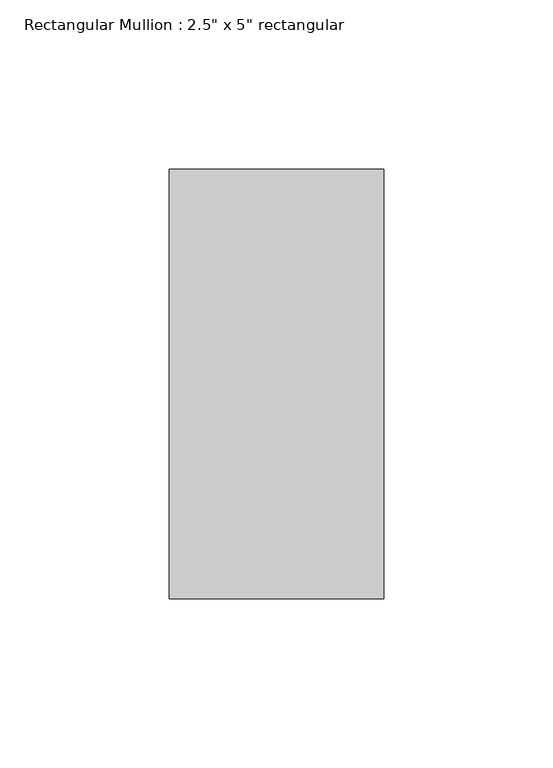
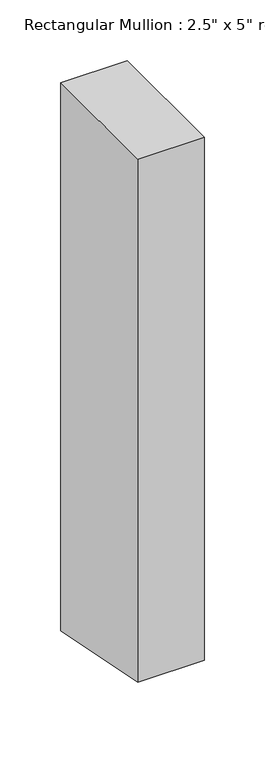
"""IFC4 building model written with IfcOpenShell, lengths in millimetres: member geometry."""

from ifc_helpers import new_model, si_unit, frame, origin, place, context, project, spatial, polyline, outline, extrude, source, transform, mapped, element, save


def member_efc2c738(model_context):
    return source(origin(), model_context, "Body", "SweptSolid", [
        extrude(outline(polyline([(-63.5, 0.0), (63.5, 0.0), (63.5, -552.0583104), (-63.5, -526.7964398), (-63.5, 0.0)])), frame((-63.5, 0.0, 0.0), z_axis=(1.0, 0.0, 0.0), x_axis=(0.0, 1.0, 0.0)), (0.0, 0.0, 1.0), 63.5),
    ])


if __name__ == "__main__":
    model = new_model("IFC4")
    model_context = context("Model", 3, world=origin())
    ifc_project = project(units=[si_unit("LENGTHUNIT", "METRE", prefix="MILLI")], contexts=[model_context])
    site = spatial("IfcSite", under=ifc_project)
    building = spatial("IfcBuilding", under=site)
    placement = place(None, origin())
    member_shape = member_efc2c738(model_context)
    element("IfcMember", 1, ObjectType="Rectangular Mullion : 2.5\" x 5\" rectangular", at=placement, inside=building, context=model_context, shape_type="MappedRepresentation", body=[
        mapped(member_shape, transform((0.0, 0.0, 0.0), x_axis=(1.0, 0.0, 0.0), y_axis=(0.0, 1.0, 0.0), z_axis=(0.0, 0.0, 1.0))),
    ])
    save(model, "model.ifc")

# Revit data of these elements
# Type "Rectangular Mullion : 2.5\" x 5\" rectangular"
#   built-in parameter 1007304 = 0.416667 (stored number, unit not read)
#   built-in parameter 1007301 = 0.104167 (stored number, unit not read)
#   built-in parameter 1007300 = 0.104167 (stored number, unit not read)
# Element 1 (IfcMember, "Rectangular Mullion : 2.5\" x 5\" rectangular")
#   Materials on its faces: "Iron, Ductile"
# Materials
#   "Iron, Ductile": class "Metal", colour RGB 0 0 0, transparency 0, Description = "Ductile cast iron", Cost = 0
